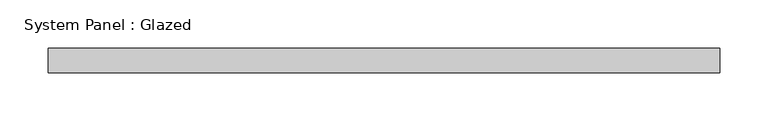
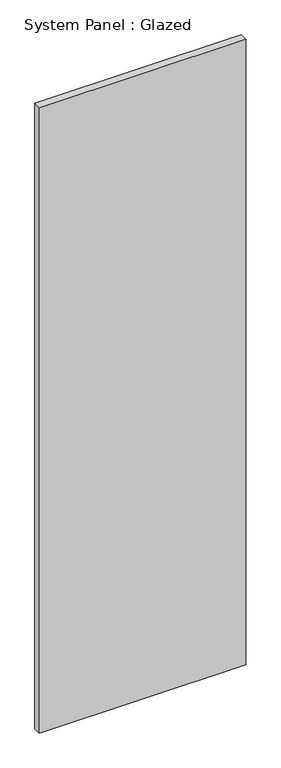
"""IFC4 building model written with IfcOpenShell, lengths in millimetres: plate geometry, System Panel : Glazed."""

from ifc_helpers import new_model, si_unit, origin, origin_with_axes, place, context, project, spatial, polyline, outline, extrude, source, transform, mapped, element, save


def system_panel_glazed_30f93ba9(model_context):
    return source(origin(), model_context, "Body", "SweptSolid", [
        extrude(outline(polyline([(349.25, 19.05), (-349.25, 19.05), (-349.25, 44.45), (349.25, 44.45), (349.25, 19.05)])), origin_with_axes(), (0.0, 0.0, 1.0), 2237.5663272),
    ])


if __name__ == "__main__":
    model = new_model("IFC4")
    model_context = context("Model", 3, world=origin())
    ifc_project = project(units=[si_unit("LENGTHUNIT", "METRE", prefix="MILLI")], contexts=[model_context])
    site = spatial("IfcSite", under=ifc_project)
    building = spatial("IfcBuilding", under=site)
    placement = place(None, origin())
    system_panel_glazed_shape = system_panel_glazed_30f93ba9(model_context)
    element("IfcPlate", 1, ObjectType="System Panel : Glazed", at=placement, inside=building, context=model_context, shape_type="MappedRepresentation", body=[
        mapped(system_panel_glazed_shape, transform((0.0, 0.0, 0.0), x_axis=(1.0, 0.0, 0.0), y_axis=(0.0, 1.0, 0.0), z_axis=(0.0, 0.0, 1.0))),
    ])
    save(model, "model.ifc")

# Revit data of these elements
# Type "System Panel : Glazed"
#   Construction Type Id = "GSP4R"
#   Analytic Construction = "1/8 in Pilkington single glazing"
#   Visual Light Transmittance = 0.9
#   Solar Heat Gain Coefficient = 0.86
#   Heat Transfer Coefficient (U) = 1.18115 BTU/(h·ft²·°F)
#   Define Thermal Properties by = 1
# Element 1 (IfcPlate, "System Panel : Glazed")
#   Materials on its faces: "Glass"
# Materials
#   "Glass": class "Glass", colour RGB 0 128 192, transparency 0.75, Description = "Soda Lime Glass", Cost = 0
